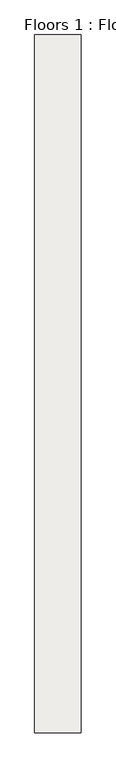
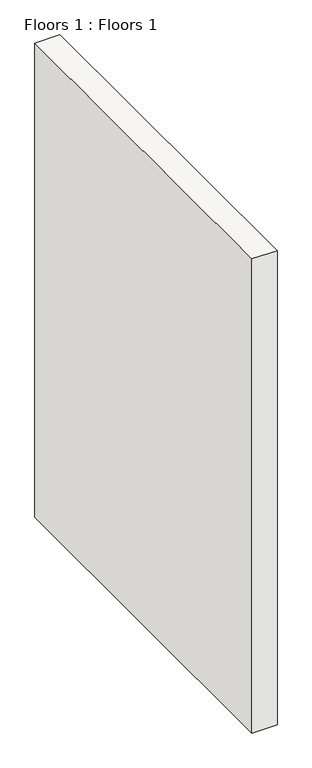
"""IFC4 building model written with IfcOpenShell, lengths in millimetres: slab geometry, Floors 1 : Floors 1."""

from ifc_helpers import new_model, si_unit, frame, origin, place, context, project, spatial, polyline, outline, extrude, source, transform, mapped, element, save


def floors_1_floors_1_82467aff(model_context):
    return source(origin(), model_context, "Body", "SweptSolid", [
        extrude(outline(polyline([(-3518.9453131, -6558.2938352), (-3518.9453131, -4272.2938352), (-3366.5453131, -4272.2938352), (-3366.5453131, -6558.2938352), (-3518.9453131, -6558.2938352)])), frame((0.0, 0.0, 3352.8), z_axis=(0.0, 0.0, 1.0), x_axis=(1.0, 0.0, 0.0)), (0.0, 0.0, 1.0), 3048.0),
    ])


if __name__ == "__main__":
    model = new_model("IFC4")
    model_context = context("Model", 3, world=origin())
    ifc_project = project(units=[si_unit("LENGTHUNIT", "METRE", prefix="MILLI")], contexts=[model_context])
    site = spatial("IfcSite", under=ifc_project)
    building = spatial("IfcBuilding", under=site)
    placement = place(None, origin())
    floors_1_floors_1_shape = floors_1_floors_1_82467aff(model_context)
    element("IfcSlab", 1, ObjectType="Floors 1 : Floors 1", at=placement, inside=building, context=model_context, shape_type="MappedRepresentation", body=[
        mapped(floors_1_floors_1_shape, transform((0.0, 0.0, 0.0), x_axis=(1.0, 0.0, 0.0), y_axis=(0.0, 1.0, 0.0), z_axis=(0.0, 0.0, 1.0))),
    ])
    save(model, "model.ifc")

# Revit data of these elements
# Element 1 (IfcSlab, "Floors 1 : Floors 1")
#   Materials on its faces: "WALL PAINT"
# Materials
#   "WALL PAINT": class "Generic", colour RGB 120 120 120, transparency 0, Cost = 0
